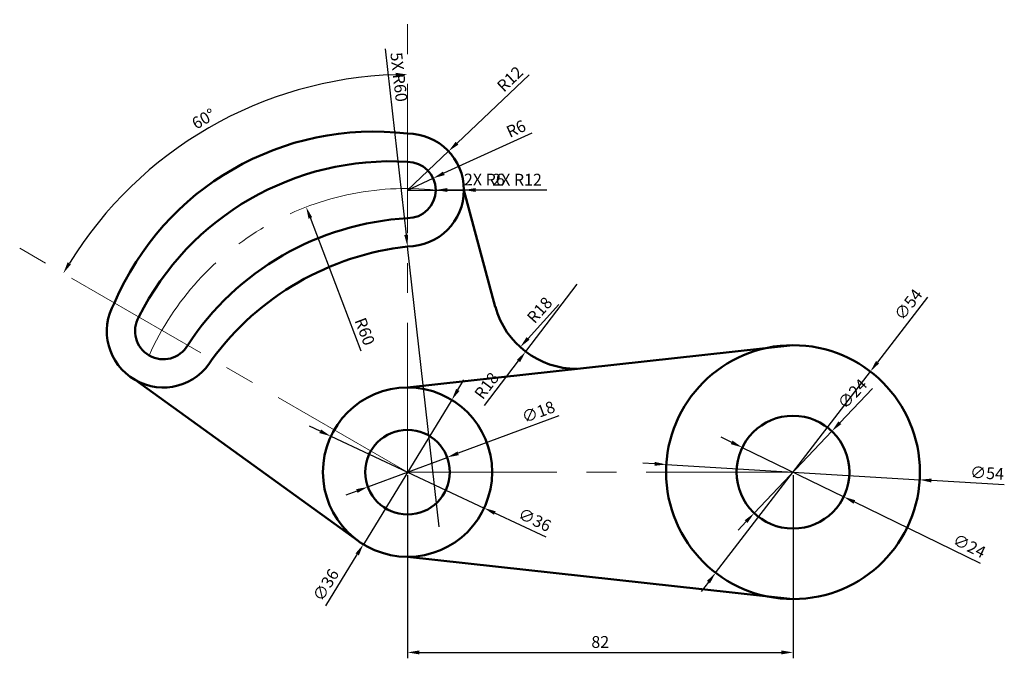
# Model space of a CAD drawing. Units: millimetres. Extents: x 2628 to 2837, y 1372 to 1508.
import ezdxf

# ---------------------------------------------------------------- set-up
doc = ezdxf.new("R2010")
doc.units = ezdxf.units.MM
doc.linetypes.add('CENTER', pattern=[50.8, 31.75, -6.35, 6.35, -6.35])
for name, color, linetype, lineweight in [('M-CNTR', 4, 'CENTER', 18), ('M-DIMS', 2, 'Continuous', 25), ('M-OUTL', 7, 'Continuous', 50)]:
    doc.layers.add(name, color=color, linetype=linetype, lineweight=lineweight)
doc.styles.get("Standard").update_dxf_attribs({"font": 'arial.ttf'})
doc.dimstyles.new('ISO-25', dxfattribs={"dimtxt": 2.5, "dimasz": 2.5, "dimexe": 1.25, "dimexo": 0.625, "dimtad": 1, "dimtxsty": 'Standard', "dimcen": 2.5, "dimadec": 0, "dimazin": 0, "dimtfac": 1, "dimtmove": 0, "dimatfit": 3, "dimfxl": 1, "dimarcsym": 0})

# ---------------------------------------------------------------- blocks, each defined once
blk = doc.blocks.new('*D1')
at = {"layer": 'Defpoints', "color": 0, "transparency": 16777216}
for p in [(2710.54, 1411.39), (2792.54, 1411.39), (2792.54, 1373.06)]:
    blk.add_point(p, dxfattribs=at)
at = {"layer": 'M-DIMS', "color": 0, "lineweight": -2, "transparency": 16777216}
for p, q in [((2710.54, 1410.77), (2710.54, 1371.81)), ((2792.54, 1410.77), (2792.54, 1371.81)), ((2713.04, 1373.06), (2790.04, 1373.06))]:
    blk.add_line(p, q, dxfattribs=at)
at = {"layer": 'M-DIMS', "color": 0, "transparency": 16777216}
for points in [[(2713.04, 1373.48), (2713.04, 1372.64), (2710.54, 1373.06)], [(2790.04, 1373.48), (2790.04, 1372.64), (2792.54, 1373.06)]]:
    blk.add_solid(points, dxfattribs=at)
at = {"layer": 'M-DIMS', "color": 0, "transparency": 16777216, "insert": (2751.54, 1374.96), "char_height": 2.5, "attachment_point": 5}
blk.add_mtext('82', dxfattribs=at)
blk = doc.blocks.new('*D2')
at = {"layer": 'Defpoints', "color": 0, "transparency": 16777216}
for p in [(2746.57, 1451.35), (2734.51, 1437.98)]:
    blk.add_point(p, dxfattribs=at)
at = {"layer": 'M-DIMS', "color": 0, "lineweight": -2, "transparency": 16777216}
blk.add_line((2742.7, 1447.06), (2736.18, 1439.84), dxfattribs=at)
at = {"layer": 'M-DIMS', "color": 0, "transparency": 16777216}
blk.add_solid([(2735.87, 1440.12), (2736.49, 1439.56), (2734.51, 1437.98)], dxfattribs=at)
at = {"layer": 'M-DIMS', "color": 0, "transparency": 16777216, "insert": (2738.87, 1445.65), "char_height": 2.5, "attachment_point": 5, "rotation": 47.9403}
blk.add_mtext('R18', dxfattribs=at)
blk = doc.blocks.new('*D3')
at = {"layer": 'Defpoints', "color": 0, "transparency": 16777216}
for p in [(2719.26, 1479.63), (2710.54, 1471.39)]:
    blk.add_point(p, dxfattribs=at)
at = {"layer": 'M-DIMS', "color": 0, "lineweight": -2, "transparency": 16777216}
for p, q in [((2736.45, 1495.88), (2721.08, 1481.35)), ((2710.54, 1471.39), (2719.26, 1479.63))]:
    blk.add_line(p, q, dxfattribs=at)
at = {"layer": 'M-DIMS', "color": 0, "transparency": 16777216}
blk.add_solid([(2720.79, 1481.65), (2721.36, 1481.05), (2719.26, 1479.63)], dxfattribs=at)
at = {"layer": 'M-DIMS', "color": 0, "transparency": 16777216, "insert": (2732.55, 1494.77), "char_height": 2.5, "attachment_point": 5, "rotation": 43.3754}
blk.add_mtext('R12', dxfattribs=at)
blk = doc.blocks.new('*D4')
at = {"layer": 'Defpoints', "color": 0, "transparency": 16777216}
for p in [(2715.99, 1473.89), (2710.54, 1471.39)]:
    blk.add_point(p, dxfattribs=at)
at = {"layer": 'M-DIMS', "color": 0, "lineweight": -2, "transparency": 16777216}
for p, q in [((2736.95, 1483.5), (2718.26, 1474.94)), ((2710.54, 1471.39), (2715.99, 1473.89))]:
    blk.add_line(p, q, dxfattribs=at)
at = {"layer": 'M-DIMS', "color": 0, "transparency": 16777216}
blk.add_solid([(2718.09, 1475.31), (2718.44, 1474.56), (2715.99, 1473.89)], dxfattribs=at)
at = {"layer": 'M-DIMS', "color": 0, "transparency": 16777216, "insert": (2733.76, 1484.13), "char_height": 2.5, "attachment_point": 5, "rotation": 24.6324}
blk.add_mtext('R6', dxfattribs=at)
blk = doc.blocks.new('*D5')
at = {"layer": 'Defpoints', "color": 0, "transparency": 16777216}
for p in [(2688.98, 1467.77), (2710.35, 1411.71)]:
    blk.add_point(p, dxfattribs=at)
at = {"layer": 'M-DIMS', "color": 0, "lineweight": -2, "transparency": 16777216}
blk.add_line((2700.66, 1437.14), (2689.87, 1465.44), dxfattribs=at)
at = {"layer": 'M-DIMS', "color": 0, "transparency": 16777216}
blk.add_solid([(2690.26, 1465.59), (2689.48, 1465.29), (2688.98, 1467.77)], dxfattribs=at)
at = {"layer": 'M-DIMS', "color": 0, "transparency": 16777216, "insert": (2701.15, 1441.19), "char_height": 2.5, "attachment_point": 5, "rotation": 290.8728}
blk.add_mtext('R60', dxfattribs=at)
blk = doc.blocks.new('*D6')
at = {"layer": 'Defpoints', "color": 0, "transparency": 16777216}
for p in [(2781.74, 1416.64), (2803.33, 1406.15)]:
    blk.add_point(p, dxfattribs=at)
at = {"layer": 'M-DIMS', "color": 0, "lineweight": -2, "transparency": 16777216}
for p, q in [((2779.5, 1417.73), (2777.25, 1418.82)), ((2781.74, 1416.64), (2803.33, 1406.15)), ((2832.45, 1392), (2805.58, 1405.06))]:
    blk.add_line(p, q, dxfattribs=at)
at = {"layer": 'M-DIMS', "color": 0, "transparency": 16777216}
for points in [[(2779.68, 1418.1), (2779.31, 1417.35), (2781.74, 1416.64)], [(2805.76, 1405.43), (2805.4, 1404.68), (2803.33, 1406.15)]]:
    blk.add_solid(points, dxfattribs=at)
at = {"layer": 'M-DIMS', "color": 0, "transparency": 16777216, "insert": (2829.92, 1395.42), "char_height": 2.5, "attachment_point": 5, "rotation": 334.0897}
blk.add_mtext('∅24', dxfattribs=at)
blk = doc.blocks.new('*D7')
at = {"layer": 'Defpoints', "color": 0, "transparency": 16777216}
for p in [(2765.59, 1413.02), (2819.49, 1409.77)]:
    blk.add_point(p, dxfattribs=at)
at = {"layer": 'M-DIMS', "color": 0, "lineweight": -2, "transparency": 16777216}
for p, q in [((2763.09, 1413.17), (2760.6, 1413.32)), ((2765.59, 1413.02), (2819.49, 1409.77)), ((2837.44, 1408.69), (2821.98, 1409.62))]:
    blk.add_line(p, q, dxfattribs=at)
at = {"layer": 'M-DIMS', "color": 0, "transparency": 16777216}
for points in [[(2763.12, 1413.58), (2763.07, 1412.75), (2765.59, 1413.02)], [(2822.01, 1410.03), (2821.96, 1409.2), (2819.49, 1409.77)]]:
    blk.add_solid(points, dxfattribs=at)
at = {"layer": 'M-DIMS', "color": 0, "transparency": 16777216, "insert": (2833.8, 1410.88), "char_height": 2.5, "attachment_point": 5, "rotation": 356.5535}
blk.add_mtext('∅54', dxfattribs=at)
blk = doc.blocks.new('*D8')
at = {"layer": 'Defpoints', "color": 0, "transparency": 16777216}
for p in [(2718.97, 1414.53), (2702.1, 1408.25)]:
    blk.add_point(p, dxfattribs=at)
at = {"layer": 'M-DIMS', "color": 0, "lineweight": -2, "transparency": 16777216}
for p, q in [((2742.71, 1423.37), (2721.32, 1415.4)), ((2702.1, 1408.25), (2718.97, 1414.53)), ((2699.76, 1407.38), (2697.42, 1406.51))]:
    blk.add_line(p, q, dxfattribs=at)
at = {"layer": 'M-DIMS', "color": 0, "transparency": 16777216}
for points in [[(2721.17, 1415.79), (2721.46, 1415.01), (2718.97, 1414.53)], [(2699.61, 1407.77), (2699.91, 1406.99), (2702.1, 1408.25)]]:
    blk.add_solid(points, dxfattribs=at)
at = {"layer": 'M-DIMS', "color": 0, "transparency": 16777216, "insert": (2738.48, 1423.9), "char_height": 2.5, "attachment_point": 5, "rotation": 20.4181}
blk.add_mtext('∅18', dxfattribs=at)
blk = doc.blocks.new('*D9')
at = {"layer": 'Defpoints', "color": 0, "transparency": 16777216}
for p in [(2719.94, 1426.74), (2701.14, 1396.04)]:
    blk.add_point(p, dxfattribs=at)
at = {"layer": 'M-DIMS', "color": 0, "lineweight": -2, "transparency": 16777216}
for p, q in [((2721.24, 1428.88), (2722.55, 1431.01)), ((2719.94, 1426.74), (2701.14, 1396.04)), ((2693.14, 1382.97), (2699.83, 1393.91))]:
    blk.add_line(p, q, dxfattribs=at)
at = {"layer": 'M-DIMS', "color": 0, "transparency": 16777216}
for points in [[(2720.89, 1429.09), (2721.6, 1428.66), (2719.94, 1426.74)], [(2699.48, 1394.13), (2700.19, 1393.69), (2701.14, 1396.04)]]:
    blk.add_solid(points, dxfattribs=at)
at = {"layer": 'M-DIMS', "color": 0, "transparency": 16777216, "insert": (2693.43, 1387.22), "char_height": 2.5, "attachment_point": 5, "rotation": 58.5198}
blk.add_mtext('∅36', dxfattribs=at)
blk = doc.blocks.new('*D10')
at = {"layer": 'Defpoints', "color": 0, "transparency": 16777216}
for p in [(2710.54, 1507.61), (2681.62, 1490.84), (2628.04, 1459.02), (2710.54, 1411.39), (2710.54, 1411.39)]:
    blk.add_point(p, dxfattribs=at)
at = {"layer": 'M-DIMS', "color": 0, "lineweight": -2, "transparency": 16777216}
blk.add_arc((2710.54, 1411.39), 84.55, 91.6942, 148.3058, dxfattribs=at)
at = {"layer": 'M-DIMS', "color": 0, "transparency": 16777216}
for points in [[(2708.03, 1496.32), (2708.04, 1495.49), (2710.54, 1495.94)], [(2638.95, 1455.6), (2638.24, 1456.03), (2637.31, 1453.67)]]:
    blk.add_solid(points, dxfattribs=at)
at = {"layer": 'M-DIMS', "color": 0, "transparency": 16777216, "insert": (2667.31, 1486.26), "char_height": 2.5, "attachment_point": 5, "rotation": 30}
blk.add_mtext('60°', dxfattribs=at)
blk = doc.blocks.new('*D11')
at = {"layer": 'Defpoints', "color": 0, "transparency": 16777216}
for p in [(2710.54, 1471.39), (2722.54, 1471.39)]:
    blk.add_point(p, dxfattribs=at)
at = {"layer": 'M-DIMS', "color": 0, "lineweight": -2, "transparency": 16777216}
for p, q in [((2710.54, 1471.39), (2722.54, 1471.39)), ((2740.15, 1471.39), (2725.04, 1471.39))]:
    blk.add_line(p, q, dxfattribs=at)
at = {"layer": 'M-DIMS', "color": 0, "transparency": 16777216}
blk.add_solid([(2725.04, 1471.81), (2725.04, 1470.98), (2722.54, 1471.39)], dxfattribs=at)
at = {"layer": 'M-DIMS', "color": 0, "transparency": 16777216, "insert": (2733.84, 1473.27), "char_height": 2.5, "attachment_point": 5, "rotation": 359.9981}
blk.add_mtext('2X R12', dxfattribs=at)
blk = doc.blocks.new('*D12')
at = {"layer": 'Defpoints', "color": 0, "transparency": 16777216}
for p in [(2710.54, 1471.39), (2716.54, 1471.39)]:
    blk.add_point(p, dxfattribs=at)
at = {"layer": 'M-DIMS', "color": 0, "lineweight": -2, "transparency": 16777216}
for p, q in [((2710.54, 1471.39), (2716.54, 1471.39)), ((2732.23, 1471.39), (2719.04, 1471.39))]:
    blk.add_line(p, q, dxfattribs=at)
at = {"layer": 'M-DIMS', "color": 0, "transparency": 16777216}
blk.add_solid([(2719.04, 1471.81), (2719.04, 1470.98), (2716.54, 1471.39)], dxfattribs=at)
at = {"layer": 'M-DIMS', "color": 0, "transparency": 16777216, "insert": (2726.88, 1473.29), "char_height": 2.5, "attachment_point": 5, "rotation": 359.9962}
blk.add_mtext('2X R6', dxfattribs=at)
blk = doc.blocks.new('*D13')
at = {"layer": 'Defpoints', "color": 0, "transparency": 16777216}
for p in [(2710.53, 1459.39), (2717.25, 1399.77)]:
    blk.add_point(p, dxfattribs=at)
at = {"layer": 'M-DIMS', "color": 0, "lineweight": -2, "transparency": 16777216}
for p, q in [((2705.79, 1501.42), (2710.25, 1461.88)), ((2717.25, 1399.77), (2710.53, 1459.39))]:
    blk.add_line(p, q, dxfattribs=at)
at = {"layer": 'M-DIMS', "color": 0, "transparency": 16777216}
blk.add_solid([(2710.66, 1461.92), (2709.84, 1461.83), (2710.53, 1459.39)], dxfattribs=at)
at = {"layer": 'M-DIMS', "color": 0, "transparency": 16777216, "insert": (2708.39, 1495.38), "char_height": 2.5, "attachment_point": 5, "rotation": 276.4291}
blk.add_mtext('5X R60', dxfattribs=at)
blk = doc.blocks.new('*D14')
at = {"layer": 'Defpoints', "color": 0, "transparency": 16777216}
for p in [(2746.57, 1451.35), (2735.66, 1437.02)]:
    blk.add_point(p, dxfattribs=at)
at = {"layer": 'M-DIMS', "color": 0, "lineweight": -2, "transparency": 16777216}
for p, q in [((2746.57, 1451.35), (2735.66, 1437.02)), ((2726.93, 1425.56), (2734.15, 1435.04))]:
    blk.add_line(p, q, dxfattribs=at)
at = {"layer": 'M-DIMS', "color": 0, "transparency": 16777216}
blk.add_solid([(2733.82, 1435.29), (2734.48, 1434.78), (2735.66, 1437.02)], dxfattribs=at)
at = {"layer": 'M-DIMS', "color": 0, "transparency": 16777216, "insert": (2727.61, 1429.58), "char_height": 2.5, "attachment_point": 5, "rotation": 52.7118}
blk.add_mtext('R18', dxfattribs=at)
blk = doc.blocks.new('*D15')
at = {"layer": 'Defpoints', "color": 0, "transparency": 16777216}
for p in [(2809, 1432.8), (2776.08, 1389.99)]:
    blk.add_point(p, dxfattribs=at)
at = {"layer": 'M-DIMS', "color": 0, "lineweight": -2, "transparency": 16777216}
for p, q in [((2821.17, 1448.63), (2810.52, 1434.78)), ((2776.08, 1389.99), (2809, 1432.8)), ((2774.55, 1388.01), (2773.03, 1386.03))]:
    blk.add_line(p, q, dxfattribs=at)
at = {"layer": 'M-DIMS', "color": 0, "transparency": 16777216}
for points in [[(2810.19, 1435.03), (2810.85, 1434.52), (2809, 1432.8)], [(2774.22, 1388.26), (2774.88, 1387.75), (2776.08, 1389.99)]]:
    blk.add_solid(points, dxfattribs=at)
at = {"layer": 'M-DIMS', "color": 0, "transparency": 16777216, "insert": (2817.31, 1446.84), "char_height": 2.5, "attachment_point": 5, "rotation": 52.4399}
blk.add_mtext('∅54', dxfattribs=at)
blk = doc.blocks.new('*D16')
at = {"layer": 'Defpoints', "color": 0, "transparency": 16777216}
for p in [(2800.8, 1420.1), (2784.28, 1402.69)]:
    blk.add_point(p, dxfattribs=at)
at = {"layer": 'M-DIMS', "color": 0, "lineweight": -2, "transparency": 16777216}
for p, q in [((2809.43, 1429.19), (2802.52, 1421.91)), ((2784.28, 1402.69), (2800.8, 1420.1)), ((2782.56, 1400.87), (2780.84, 1399.06))]:
    blk.add_line(p, q, dxfattribs=at)
at = {"layer": 'M-DIMS', "color": 0, "transparency": 16777216}
for points in [[(2802.22, 1422.2), (2802.82, 1421.62), (2800.8, 1420.1)], [(2782.25, 1401.16), (2782.86, 1400.59), (2784.28, 1402.69)]]:
    blk.add_solid(points, dxfattribs=at)
at = {"layer": 'M-DIMS', "color": 0, "transparency": 16777216, "insert": (2805.4, 1427.82), "char_height": 2.5, "attachment_point": 5, "rotation": 46.5029}
blk.add_mtext('∅24', dxfattribs=at)
blk = doc.blocks.new('*D17')
at = {"layer": 'Defpoints', "color": 0, "transparency": 16777216}
for p in [(2694.24, 1419.02), (2726.84, 1403.76)]:
    blk.add_point(p, dxfattribs=at)
at = {"layer": 'M-DIMS', "color": 0, "lineweight": -2, "transparency": 16777216}
for p, q in [((2691.97, 1420.08), (2689.71, 1421.14)), ((2694.24, 1419.02), (2726.84, 1403.76)), ((2740.04, 1397.58), (2729.1, 1402.7))]:
    blk.add_line(p, q, dxfattribs=at)
at = {"layer": 'M-DIMS', "color": 0, "transparency": 16777216}
for points in [[(2692.15, 1420.46), (2691.79, 1419.71), (2694.24, 1419.02)], [(2729.28, 1403.08), (2728.93, 1402.32), (2726.84, 1403.76)]]:
    blk.add_solid(points, dxfattribs=at)
at = {"layer": 'M-DIMS', "color": 0, "transparency": 16777216, "insert": (2737.46, 1400.97), "char_height": 2.5, "attachment_point": 5, "rotation": 334.9121}
blk.add_mtext('∅36', dxfattribs=at)

msp = doc.modelspace()

# ---------------------------------------------------------------- linework, layer by layer
at = {"layer": 'M-CNTR'}
for q in [(2710.538, 1507.607), (2628.038, 1459.023), (2792.538, 1411.392)]:
    msp.add_line((2710.538, 1411.392), q, dxfattribs=at)
msp.add_arc((2710.353, 1411.712), 60, 84.08372, 155.91628, dxfattribs=at)
at = {"layer": 'M-OUTL'}
for p, q in [((2722.538, 1471.392), (2729.218, 1446.546)), ((2710.538, 1429.392), (2792.538, 1438.392)), ((2652.576, 1431), (2700.009, 1396.793)), ((2710.538, 1393.392), (2792.538, 1384.392))]:
    msp.add_line(p, q, dxfattribs=at)
for centre, radius in [((2792.538, 1411.392), 27), ((2710.538, 1411.392), 18), ((2792.538, 1411.392), 12), ((2710.538, 1411.392), 9)]:
    msp.add_circle(centre, radius, dxfattribs=at)
for centre, radius, start, end in [((2703.361, 1423.823), 60, 83.1301, 156.8699), ((2710.538, 1471.392), 12, 270, 90), ((2707.014, 1417.496), 60, 86.63299, 153.36701), ((2710.538, 1471.392), 6, 270, 90), ((2713.946, 1405.489), 60, 93.25632, 146.74368), ((2717.248, 1399.769), 60, 96.42182, 143.57818), ((2658.576, 1441.392), 12, 150, 330), ((2746.567, 1451.345), 18, 195.46513, 269.95782), ((2658.576, 1441.392), 6, 150, 330)]:
    msp.add_arc(centre, radius, start, end, dxfattribs=at)

# ---------------------------------------------------------------- dimensions: what is measured, and where the dimension line sits
at = {"layer": 'M-DIMS'}
dim = msp.add_angular_dim_2l(base=(2681.619, 1490.845), line1=((2710.538, 1411.392), (2710.538, 1507.607)), line2=((2710.538, 1411.392), (2628.038, 1459.023)), dimstyle='ISO-25', override={"dimclrd": 0, "dimclre": 0, "dimclrt": 0}, dxfattribs=at)
dim.commit()
dim.dimension.update_dxf_attribs({"geometry": '*D10', "text_midpoint": (2667.311, 1486.263)})
dim = msp.add_radius_dim(center=(2717.248, 1399.769), mpoint=(2710.53, 1459.392), text='5X <>', dimstyle='ISO-25', override={"dimdec": 0, "dimlfac": 1, "dimrnd": 0, "dimzin": 0, "dimdsep": 46, "dimlunit": 2}, dxfattribs=at)
dim.commit()
dim.dimension.update_dxf_attribs({"geometry": '*D13', "text_midpoint": (2706.499, 1495.165), "dimtype": 164})
for center, mpoint, override, picture, middle in [((2710.538, 1471.392), (2719.26, 1479.634), {"dimclrd": 0, "dimclre": 0, "dimclrt": 0}, '*D3', (2733.837, 1493.407)), ((2710.538, 1471.392), (2715.992, 1473.893), {"dimclrd": 0, "dimclre": 0, "dimclrt": 0}, '*D4', (2734.548, 1482.402)), ((2710.353, 1411.712), (2688.975, 1467.774), {"dimclrd": 0, "dimclre": 0, "dimclrt": 0}, '*D5', (2699.372, 1440.51)), ((2746.567, 1451.345), (2735.662, 1437.025), {"dimdec": 0, "dimlfac": 1, "dimrnd": 0, "dimzin": 0, "dimdsep": 46, "dimlunit": 2}, '*D14', (2729.119, 1428.432)), ((2746.567, 1451.345), (2734.508, 1437.981), {"dimclrd": 0, "dimclre": 0, "dimclrt": 0}, '*D2', (2740.279, 1444.377))]:
    dim = msp.add_radius_dim(center=center, mpoint=mpoint, dimstyle='ISO-25', override=override, dxfattribs=at)
    dim.commit()
    dim.dimension.update_dxf_attribs({"geometry": picture, "text_midpoint": middle, "dimtype": 164})
for mpoint, picture, middle in [((2716.538, 1471.392), '*D12', (2726.885, 1473.293)), ((2722.538, 1471.392), '*D11', (2733.844, 1473.273))]:
    dim = msp.add_radius_dim(center=(2710.538, 1471.392), mpoint=mpoint, text='2X <>', dimstyle='ISO-25', override={"dimdec": 0, "dimlfac": 1, "dimrnd": 0, "dimzin": 0, "dimdsep": 46, "dimlunit": 2}, dxfattribs=at)
    dim.commit()
    dim.dimension.update_dxf_attribs({"geometry": picture, "text_midpoint": middle})
for p1, p2, override, picture, middle in [((2776.079, 1389.989), (2808.997, 1432.796), {"dimdec": 0, "dimlfac": 1, "dimrnd": 0, "dimzin": 0, "dimdsep": 46, "dimlunit": 2}, '*D15', (2818.872, 1445.638)), ((2719.937, 1426.743), (2701.138, 1396.042), {"dimclrd": 0, "dimclre": 0, "dimclrt": 0}, '*D9', (2695.108, 1386.194)), ((2702.103, 1408.253), (2718.972, 1414.532), {"dimclrd": 0, "dimclre": 0, "dimclrt": 0}, '*D8', (2739.167, 1422.05)), ((2694.236, 1419.025), (2726.839, 1403.76), {"dimdec": 0, "dimlfac": 1, "dimrnd": 0, "dimzin": 0, "dimdsep": 46, "dimlunit": 2}, '*D17', (2736.621, 1399.181)), ((2781.744, 1416.636), (2803.331, 1406.149), {"dimclrd": 0, "dimclre": 0, "dimclrt": 0}, '*D6', (2829.062, 1393.649)), ((2765.586, 1413.016), (2819.489, 1409.769), {"dimclrd": 0, "dimclre": 0, "dimclrt": 0}, '*D7', (2833.681, 1408.915))]:
    dim = msp.add_diameter_dim_2p(p1=p1, p2=p2, dimstyle='ISO-25', override=override, dxfattribs=at)
    dim.commit()
    dim.dimension.update_dxf_attribs({"geometry": picture, "text_midpoint": middle, "dimtype": 163})
dim = msp.add_diameter_dim_2p(p1=(2784.278, 1402.687), p2=(2800.797, 1420.097), dimstyle='ISO-25', override={"dimdec": 0, "dimlfac": 1, "dimrnd": 0, "dimzin": 0, "dimdsep": 46, "dimlunit": 2}, dxfattribs=at)
dim.commit()
dim.dimension.update_dxf_attribs({"geometry": '*D16', "text_midpoint": (2806.834, 1426.459)})
dim = msp.add_linear_dim(base=(2792.538, 1373.059), p1=(2710.538, 1411.392), p2=(2792.538, 1411.392), dimstyle='ISO-25', override={"dimclrd": 0, "dimclre": 0, "dimclrt": 0}, dxfattribs=at)
dim.commit()
dim.dimension.update_dxf_attribs({"geometry": '*D1', "text_midpoint": (2751.538, 1374.96)})

doc.saveas('drawing.dxf')
